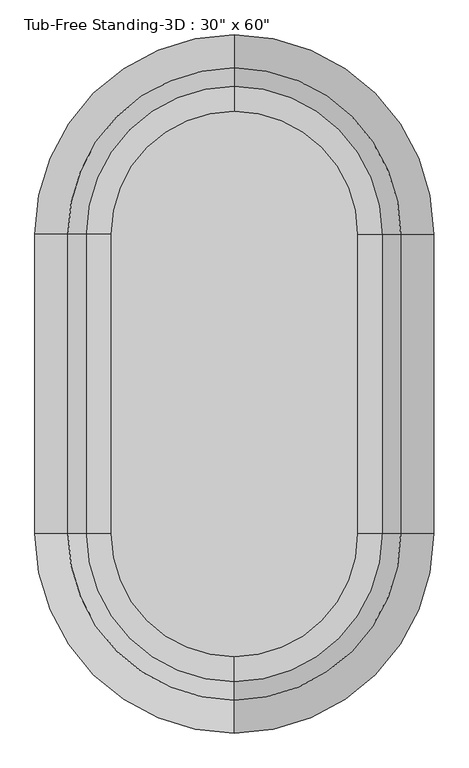
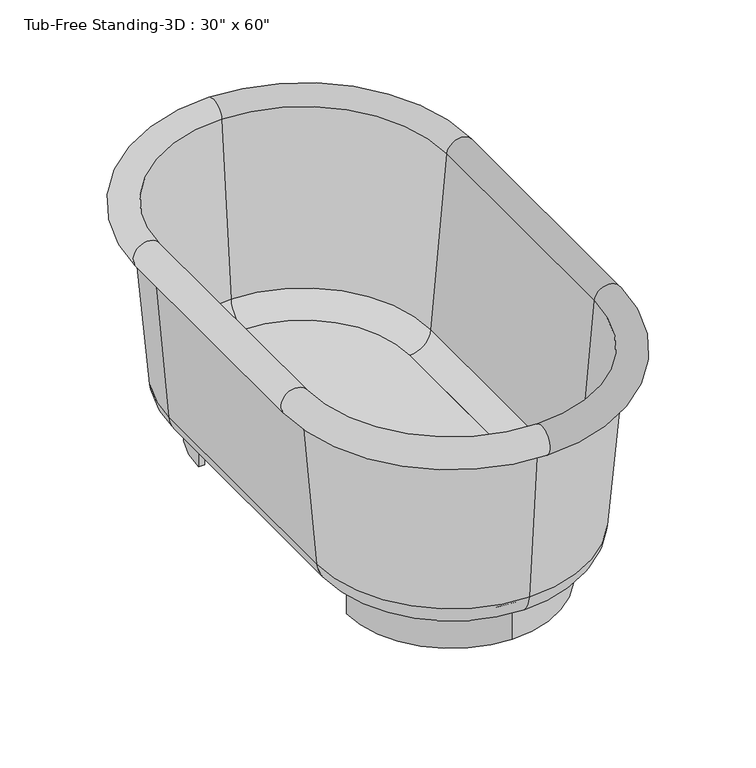
"""IFC4 building model written with IfcOpenShell, lengths in millimetres: flow terminal geometry."""

from ifc_helpers import new_model, si_unit, point, frame, frame_2d, origin, origin_with_axes, place, context, project, spatial, polyline, circle_curve, ellipse_curve, trimmed, segment, composite_curve, outline, extrude, source, transform, mapped, element, save
from ifc_brep_helpers import plane_surface, cylinder_surface, revolved_surface, advanced_brep


def flow_terminal_f143e1fa(model_context):
    return source(origin(), model_context, "Body", "SolidModel", [
        extrude(outline(composite_curve([segment(trimmed(circle_curve(frame_2d((0.0, 228.6)), 177.8), [point((0.0, 406.4))], [point((-177.8, 228.6))], True, "CARTESIAN"), True, "CONTINUOUS"), segment(polyline([(-177.8, 228.6), (-188.0824236, 228.6)]), True, "CONTINUOUS"), segment(trimmed(circle_curve(frame_2d((0.0, 228.6)), 188.0824236), [point((-188.0824236, 228.6))], [point((0.0, 416.6824236))], False, "CARTESIAN"), True, "CONTINUOUS"), segment(trimmed(circle_curve(frame_2d((0.0, 228.6)), 188.0824236), [point((0.0, 416.6824236))], [point((188.0824236, 228.6))], False, "CARTESIAN"), True, "CONTINUOUS"), segment(polyline([(188.0824236, 228.6), (177.8, 228.6)]), True, "CONTINUOUS"), segment(trimmed(circle_curve(frame_2d((0.0, 228.6)), 177.8), [point((177.8, 228.6))], [point((0.0, 406.4))], True, "CARTESIAN"), True, "CONTINUOUS")], self_intersect=False)), origin_with_axes(), (0.0, 0.0, 1.0), 63.5),
        extrude(outline(composite_curve([segment(trimmed(circle_curve(frame_2d((0.0, -228.6)), 188.0824236), [point((0.0, -416.6824236))], [point((-188.0824236, -228.6))], False, "CARTESIAN"), True, "CONTINUOUS"), segment(polyline([(-188.0824236, -228.6), (-177.8, -228.6)]), True, "CONTINUOUS"), segment(trimmed(circle_curve(frame_2d((0.0, -228.6)), 177.8), [point((-177.8, -228.6))], [point((0.0, -406.4))], True, "CARTESIAN"), True, "CONTINUOUS"), segment(trimmed(circle_curve(frame_2d((0.0, -228.6)), 177.8), [point((0.0, -406.4))], [point((177.8, -228.6))], True, "CARTESIAN"), True, "CONTINUOUS"), segment(polyline([(177.8, -228.6), (188.0824236, -228.6)]), True, "CONTINUOUS"), segment(trimmed(circle_curve(frame_2d((0.0, -228.6)), 188.0824236), [point((188.0824236, -228.6))], [point((0.0, -416.6824236))], False, "CARTESIAN"), True, "CONTINUOUS")], self_intersect=False)), origin_with_axes(), (0.0, 0.0, 1.0), 63.5),
        extrude(outline(composite_curve([segment(polyline([(-188.0824236, -228.6), (-188.0824236, 228.6)]), True, "CONTINUOUS"), segment(trimmed(circle_curve(frame_2d((0.0, 228.6)), 188.0824236), [point((-188.0824236, 228.6))], [point((0.0, 416.6824236))], False, "CARTESIAN"), True, "CONTINUOUS"), segment(trimmed(circle_curve(frame_2d((0.0, 228.6)), 188.0824236), [point((0.0, 416.6824236))], [point((188.0824236, 228.6))], False, "CARTESIAN"), True, "CONTINUOUS"), segment(polyline([(188.0824236, 228.6), (188.0824236, -228.6)]), True, "CONTINUOUS"), segment(trimmed(circle_curve(frame_2d((0.0, -228.6)), 188.0824236), [point((188.0824236, -228.6))], [point((0.0, -416.6824236))], False, "CARTESIAN"), True, "CONTINUOUS"), segment(trimmed(circle_curve(frame_2d((0.0, -228.6)), 188.0824236), [point((0.0, -416.6824236))], [point((-188.0824236, -228.6))], False, "CARTESIAN"), True, "CONTINUOUS")], self_intersect=False)), frame((0.0, 0.0, 63.5), z_axis=(0.0, 0.0, 1.0), x_axis=(1.0, 0.0, 0.0)), (0.0, 0.0, 1.0), 15.08125),
        advanced_brep(
        [(0.0, -495.3, 406.4), (266.7, -228.6, 406.4), (279.4, -228.6, 406.4), (0.0, -508.0, 406.4), (0.0, -469.5045038, 111.5561295), (240.9045038, -228.6, 111.5561295), (0.0, -416.6824236, 63.1536107), (188.0824236, -228.6, 63.1536107), (0.0, -416.6824236, 78.0774627), (188.0824236, -228.6, 78.0774627), (0.0, -454.6374416, 112.8568289), (226.0374416, -228.6, 112.8568289), (0.0, -482.8561556, 435.3982063), (254.2561556, -228.6, 435.3982063), (-266.7, -228.6, 406.4), (-279.4, -228.6, 406.4), (-240.9045038, -228.6, 111.5561295), (-188.0824236, -228.6, 63.1536107), (-188.0824236, -228.6, 78.0774627), (-226.0374416, -228.6, 112.8568289), (-254.2561556, -228.6, 435.3982063), (-279.4, 228.6, 406.4), (-266.7, 228.6, 406.4), (-240.9045038, 228.6, 111.5561295), (-188.0824236, 228.6, 63.1536107), (-188.0824236, 228.6, 78.0774627), (-226.0374416, 228.6, 112.8568289), (-254.2561556, 228.6, 435.3982063), (0.0, 495.3, 406.4), (0.0, 508.0, 406.4), (0.0, 469.5045038, 111.5561295), (0.0, 416.6824236, 63.1536107), (0.0, 416.6824236, 78.0774627), (0.0, 454.6374416, 112.8568289), (0.0, 482.8561556, 435.3982063), (266.7, 228.6, 406.4), (279.4, 228.6, 406.4), (240.9045038, 228.6, 111.5561295), (188.0824236, 228.6, 63.1536107), (188.0824236, 228.6, 78.0774627), (226.0374416, 228.6, 112.8568289), (254.2561556, 228.6, 435.3982063)],
        [
            (0, 1, circle_curve(frame((0.0, -228.6, 406.4), z_axis=(0.0, 0.0, 1.0), x_axis=(1.0, 0.0, 0.0)), 266.7)),
            (1, 2),
            (2, 3, circle_curve(frame((0.0, -228.6, 406.4), z_axis=(0.0, 0.0, -1.0), x_axis=(1.0, 0.0, 0.0)), 279.4)),
            (3, 0),
            (4, 5, circle_curve(frame((0.0, -228.6, 111.5561295), z_axis=(0.0, 0.0, 1.0), x_axis=(1.0, 0.0, 0.0)), 240.9045038)),
            (5, 1),
            (0, 4),
            (6, 7, circle_curve(frame((0.0, -228.6, 63.1536107), z_axis=(0.0, 0.0, 1.0), x_axis=(1.0, 0.0, 0.0)), 188.0824236)),
            (7, 5, circle_curve(frame((188.0824236, -228.6, 116.1774627), z_axis=(0.0, -1.0, 0.0), x_axis=(1.0, 0.0, 0.0)), 53.023852)),
            (4, 6, circle_curve(frame((0.0, -416.6824236, 116.1774627), z_axis=(1.0, 0.0, 0.0), x_axis=(0.0, -1.0, 0.0)), 53.023852)),
            (8, 9, circle_curve(frame((0.0, -228.6, 78.0774627), z_axis=(0.0, 0.0, 1.0), x_axis=(1.0, 0.0, 0.0)), 188.0824236)),
            (9, 7),
            (6, 8),
            (10, 11, circle_curve(frame((0.0, -228.6, 112.8568289), z_axis=(0.0, 0.0, 1.0), x_axis=(1.0, 0.0, 0.0)), 226.0374416)),
            (11, 9, circle_curve(frame((188.0824236, -228.6, 116.1774627), z_axis=(0.0, 1.0, 0.0), x_axis=(1.0, 0.0, 0.0)), 38.1)),
            (8, 10, circle_curve(frame((0.0, -416.6824236, 116.1774627), z_axis=(-1.0, 0.0, 0.0), x_axis=(0.0, -1.0, 0.0)), 38.1)),
            (12, 13, circle_curve(frame((0.0, -228.6, 435.3982063), z_axis=(0.0, 0.0, 1.0), x_axis=(1.0, 0.0, 0.0)), 254.2561556)),
            (13, 11),
            (10, 12),
            (2, 13, circle_curve(frame((279.4, -228.6, 431.8), z_axis=(0.0, -1.0, 0.0), x_axis=(1.0, 0.0, 0.0)), 25.4)),
            (12, 3, circle_curve(frame((0.0, -508.0, 431.8), z_axis=(1.0, 0.0, 0.0), x_axis=(0.0, -1.0, 0.0)), 25.4)),
            (14, 0, circle_curve(frame((0.0, -228.6, 406.4), z_axis=(0.0, 0.0, 1.0), x_axis=(0.0, -1.0, 0.0)), 266.7)),
            (3, 15, circle_curve(frame((0.0, -228.6, 406.4), z_axis=(0.0, 0.0, -1.0), x_axis=(0.0, -1.0, 0.0)), 279.4)),
            (15, 14),
            (16, 4, circle_curve(frame((0.0, -228.6, 111.5561295), z_axis=(0.0, 0.0, 1.0), x_axis=(0.0, -1.0, 0.0)), 240.9045038)),
            (14, 16),
            (17, 6, circle_curve(frame((0.0, -228.6, 63.1536107), z_axis=(0.0, 0.0, 1.0), x_axis=(0.0, -1.0, 0.0)), 188.0824236)),
            (16, 17, circle_curve(frame((-188.0824236, -228.6, 116.1774627), z_axis=(0.0, -1.0, 0.0), x_axis=(-1.0, 0.0, 0.0)), 53.023852)),
            (18, 8, circle_curve(frame((0.0, -228.6, 78.0774627), z_axis=(0.0, 0.0, 1.0), x_axis=(0.0, -1.0, 0.0)), 188.0824236)),
            (17, 18),
            (19, 10, circle_curve(frame((0.0, -228.6, 112.8568289), z_axis=(0.0, 0.0, 1.0), x_axis=(0.0, -1.0, 0.0)), 226.0374416)),
            (18, 19, circle_curve(frame((-188.0824236, -228.6, 116.1774627), z_axis=(0.0, 1.0, 0.0), x_axis=(-1.0, 0.0, 0.0)), 38.1)),
            (20, 12, circle_curve(frame((0.0, -228.6, 435.3982063), z_axis=(0.0, 0.0, 1.0), x_axis=(0.0, -1.0, 0.0)), 254.2561556)),
            (19, 20),
            (20, 15, circle_curve(frame((-279.4, -228.6, 431.8), z_axis=(0.0, -1.0, 0.0), x_axis=(-1.0, 0.0, 0.0)), 25.4)),
            (15, 21),
            (21, 22),
            (22, 14),
            (22, 23),
            (23, 16),
            (23, 24, circle_curve(frame((-188.0824236, 228.6, 116.1774627), z_axis=(0.0, -1.0, 0.0), x_axis=(-1.0, 0.0, 0.0)), 53.023852)),
            (24, 17),
            (24, 25),
            (25, 18),
            (25, 26, circle_curve(frame((-188.0824236, 228.6, 116.1774627), z_axis=(0.0, 1.0, 0.0), x_axis=(-1.0, 0.0, 0.0)), 38.1)),
            (26, 19),
            (26, 27),
            (27, 20),
            (27, 21, circle_curve(frame((-279.4, 228.6, 431.8), z_axis=(0.0, -1.0, 0.0), x_axis=(-1.0, 0.0, 0.0)), 25.4)),
            (28, 22, circle_curve(frame((0.0, 228.6, 406.4), z_axis=(0.0, 0.0, 1.0), x_axis=(-1.0, 0.0, 0.0)), 266.7)),
            (21, 29, circle_curve(frame((0.0, 228.6, 406.4), z_axis=(0.0, 0.0, -1.0), x_axis=(-1.0, 0.0, 0.0)), 279.4)),
            (29, 28),
            (30, 23, circle_curve(frame((0.0, 228.6, 111.5561295), z_axis=(0.0, 0.0, 1.0), x_axis=(-1.0, 0.0, 0.0)), 240.9045038)),
            (28, 30),
            (31, 24, circle_curve(frame((0.0, 228.6, 63.1536107), z_axis=(0.0, 0.0, 1.0), x_axis=(-1.0, 0.0, 0.0)), 188.0824236)),
            (30, 31, circle_curve(frame((0.0, 416.6824236, 116.1774627), z_axis=(-1.0, 0.0, 0.0), x_axis=(0.0, 1.0, 0.0)), 53.023852)),
            (32, 25, circle_curve(frame((0.0, 228.6, 78.0774627), z_axis=(0.0, 0.0, 1.0), x_axis=(-1.0, 0.0, 0.0)), 188.0824236)),
            (31, 32),
            (33, 26, circle_curve(frame((0.0, 228.6, 112.8568289), z_axis=(0.0, 0.0, 1.0), x_axis=(-1.0, 0.0, 0.0)), 226.0374416)),
            (32, 33, circle_curve(frame((0.0, 416.6824236, 116.1774627), z_axis=(1.0, 0.0, 0.0), x_axis=(0.0, 1.0, 0.0)), 38.1)),
            (34, 27, circle_curve(frame((0.0, 228.6, 435.3982063), z_axis=(0.0, 0.0, 1.0), x_axis=(-1.0, 0.0, 0.0)), 254.2561556)),
            (33, 34),
            (34, 29, circle_curve(frame((0.0, 508.0, 431.8), z_axis=(-1.0, 0.0, 0.0), x_axis=(0.0, 1.0, 0.0)), 25.4)),
            (35, 28, circle_curve(frame((0.0, 228.6, 406.4), z_axis=(0.0, 0.0, 1.0), x_axis=(0.0, 1.0, 0.0)), 266.7)),
            (29, 36, circle_curve(frame((0.0, 228.6, 406.4), z_axis=(0.0, 0.0, -1.0), x_axis=(0.0, 1.0, 0.0)), 279.4)),
            (36, 35),
            (37, 30, circle_curve(frame((0.0, 228.6, 111.5561295), z_axis=(0.0, 0.0, 1.0), x_axis=(0.0, 1.0, 0.0)), 240.9045038)),
            (35, 37),
            (38, 31, circle_curve(frame((0.0, 228.6, 63.1536107), z_axis=(0.0, 0.0, 1.0), x_axis=(0.0, 1.0, 0.0)), 188.0824236)),
            (37, 38, circle_curve(frame((188.0824236, 228.6, 116.1774627), z_axis=(0.0, 1.0, 0.0), x_axis=(1.0, 0.0, 0.0)), 53.023852)),
            (39, 32, circle_curve(frame((0.0, 228.6, 78.0774627), z_axis=(0.0, 0.0, 1.0), x_axis=(0.0, 1.0, 0.0)), 188.0824236)),
            (38, 39),
            (40, 33, circle_curve(frame((0.0, 228.6, 112.8568289), z_axis=(0.0, 0.0, 1.0), x_axis=(0.0, 1.0, 0.0)), 226.0374416)),
            (39, 40, circle_curve(frame((188.0824236, 228.6, 116.1774627), z_axis=(0.0, -1.0, 0.0), x_axis=(1.0, 0.0, 0.0)), 38.1)),
            (41, 34, circle_curve(frame((0.0, 228.6, 435.3982063), z_axis=(0.0, 0.0, 1.0), x_axis=(0.0, 1.0, 0.0)), 254.2561556)),
            (40, 41),
            (41, 36, circle_curve(frame((279.4, 228.6, 431.8), z_axis=(0.0, 1.0, 0.0), x_axis=(1.0, 0.0, 0.0)), 25.4)),
            (36, 2),
            (1, 35),
            (5, 37),
            (7, 38),
            (9, 39),
            (11, 40),
            (13, 41),
        ],
        [
            plane_surface(frame((0.0, -228.6, 406.4), z_axis=(0.0, 0.0, -1.0), x_axis=(1.0, 0.0, 0.0))),
            revolved_surface(polyline([(266.7, -228.6, 406.4), (240.9045038, -228.6, 111.5561295)]), (0.0, -228.6, 431.8), (0.0, 0.0, -1.0)),
            revolved_surface(trimmed(ellipse_curve(frame((188.0824236, -228.6, 116.1774627), z_axis=(0.0, 1.0, 0.0), x_axis=(1.0, 0.0, 0.0)), 53.023852, 53.023852), [point((240.9045038, -228.6, 111.5561295))], [point((188.0824236, -228.6, 63.1536107))], True, "CARTESIAN"), (0.0, -228.6, 431.8), (0.0, 0.0, -1.0)),
            revolved_surface(polyline([(188.0824236, -228.6, 63.1536107), (188.0824236, -228.6, 78.07746270000001)]), (0.0, -228.6, 431.8), (0.0, 0.0, -1.0)),
            revolved_surface(trimmed(ellipse_curve(frame((188.0824236, -228.6, 116.1774627), z_axis=(0.0, -1.0, 0.0), x_axis=(1.0, 0.0, 0.0)), 38.1, 38.1), [point((188.0824236, -228.6, 78.0774627))], [point((226.0374416, -228.6, 112.8568289))], True, "CARTESIAN"), (0.0, -228.6, 431.8), (0.0, 0.0, -1.0)),
            revolved_surface(polyline([(226.0374416, -228.6, 112.8568289), (254.2561556, -228.6, 435.3982063)]), (0.0, -228.6, 431.8), (0.0, 0.0, -1.0)),
            revolved_surface(trimmed(ellipse_curve(frame((279.4, -228.6, 431.8), z_axis=(0.0, 1.0, 0.0), x_axis=(1.0, 0.0, 0.0)), 25.4, 25.4), [point((254.2561556, -228.6, 435.3982063))], [point((279.4, -228.6, 406.4))], True, "CARTESIAN"), (0.0, -228.6, 431.8), (0.0, 0.0, -1.0)),
            plane_surface(frame((0.0, -228.6, 406.4), z_axis=(0.0, 0.0, -1.0), x_axis=(0.0, -1.0, 0.0))),
            revolved_surface(polyline([(0.0, -495.3, 406.4), (0.0, -469.5045038, 111.5561295)]), (0.0, -228.6, 431.8), (0.0, 0.0, -1.0)),
            revolved_surface(trimmed(ellipse_curve(frame((0.0, -416.6824236, 116.1774627), z_axis=(1.0, 0.0, 0.0), x_axis=(0.0, -1.0, 0.0)), 53.023852, 53.023852), [point((0.0, -469.5045038, 111.5561295))], [point((0.0, -416.6824236, 63.1536107))], True, "CARTESIAN"), (0.0, -228.6, 431.8), (0.0, 0.0, -1.0)),
            revolved_surface(polyline([(0.0, -416.6824236, 63.1536107), (0.0, -416.6824236, 78.07746270000001)]), (0.0, -228.6, 431.8), (0.0, 0.0, -1.0)),
            revolved_surface(trimmed(ellipse_curve(frame((0.0, -416.6824236, 116.1774627), z_axis=(-1.0, 0.0, 0.0), x_axis=(0.0, -1.0, 0.0)), 38.1, 38.1), [point((0.0, -416.6824236, 78.0774627))], [point((0.0, -454.6374416, 112.8568289))], True, "CARTESIAN"), (0.0, -228.6, 431.8), (0.0, 0.0, -1.0)),
            revolved_surface(polyline([(0.0, -454.6374416, 112.8568289), (0.0, -482.8561556, 435.3982063)]), (0.0, -228.6, 431.8), (0.0, 0.0, -1.0)),
            revolved_surface(trimmed(ellipse_curve(frame((0.0, -508.0, 431.8), z_axis=(1.0, 0.0, 0.0), x_axis=(0.0, -1.0, 0.0)), 25.4, 25.4), [point((0.0, -482.8561556, 435.3982063))], [point((0.0, -508.0, 406.4))], True, "CARTESIAN"), (0.0, -228.6, 431.8), (0.0, 0.0, -1.0)),
            plane_surface(frame((-279.4, -228.6, 406.4), z_axis=(0.0, 0.0, -1.0), x_axis=(0.0, 1.0, 0.0))),
            plane_surface(frame((-266.7, -228.6, 406.4), z_axis=(-0.9961946980917455, 0.0, -0.08715574274765882), x_axis=(0.0, 1.0, 0.0))),
            cylinder_surface(frame((-188.0824236, -228.6, 116.1774627), z_axis=(0.0, -1.0, 0.0), x_axis=(-1.0, 0.0, 0.0)), 53.023852),
            plane_surface(frame((-188.0824236, -228.6, 63.1536107), z_axis=(1.0, 0.0, 0.0), x_axis=(0.0, 1.0, 0.0))),
            revolved_surface(polyline([(-226.1824236, 228.6, 116.1774627), (-226.1824236, -228.6, 116.1774627)]), (-188.0824236, -228.6, 116.1774627), (0.0, 1.0, 0.0)),
            plane_surface(frame((-226.0374416, -228.6, 112.8568289), z_axis=(0.9961946980917457, 0.0, 0.08715574274765679), x_axis=(0.0, 1.0, 0.0))),
            cylinder_surface(frame((-279.4, -228.6, 431.8), z_axis=(0.0, -1.0, 0.0), x_axis=(-1.0, 0.0, 0.0)), 25.4),
            plane_surface(frame((0.0, 228.6, 406.4), z_axis=(0.0, 0.0, -1.0), x_axis=(-1.0, 0.0, 0.0))),
            revolved_surface(polyline([(-266.7, 228.6, 406.4), (-240.9045038, 228.6, 111.5561295)]), (0.0, 228.6, 431.8), (0.0, 0.0, -1.0)),
            revolved_surface(trimmed(ellipse_curve(frame((-188.0824236, 228.6, 116.1774627), z_axis=(0.0, -1.0, 0.0), x_axis=(-1.0, 0.0, 0.0)), 53.023852, 53.023852), [point((-240.9045038, 228.6, 111.5561295))], [point((-188.0824236, 228.6, 63.1536107))], True, "CARTESIAN"), (0.0, 228.6, 431.8), (0.0, 0.0, -1.0)),
            revolved_surface(polyline([(-188.0824236, 228.6, 63.1536107), (-188.0824236, 228.6, 78.07746270000001)]), (0.0, 228.6, 431.8), (0.0, 0.0, -1.0)),
            revolved_surface(trimmed(ellipse_curve(frame((-188.0824236, 228.6, 116.1774627), z_axis=(0.0, 1.0, 0.0), x_axis=(-1.0, 0.0, 0.0)), 38.1, 38.1), [point((-188.0824236, 228.6, 78.0774627))], [point((-226.0374416, 228.6, 112.8568289))], True, "CARTESIAN"), (0.0, 228.6, 431.8), (0.0, 0.0, -1.0)),
            revolved_surface(polyline([(-226.0374416, 228.6, 112.8568289), (-254.2561556, 228.6, 435.3982063)]), (0.0, 228.6, 431.8), (0.0, 0.0, -1.0)),
            revolved_surface(trimmed(ellipse_curve(frame((-279.4, 228.6, 431.8), z_axis=(0.0, -1.0, 0.0), x_axis=(-1.0, 0.0, 0.0)), 25.4, 25.4), [point((-254.2561556, 228.6, 435.3982063))], [point((-279.4, 228.6, 406.4))], True, "CARTESIAN"), (0.0, 228.6, 431.8), (0.0, 0.0, -1.0)),
            plane_surface(frame((0.0, 228.6, 406.4), z_axis=(0.0, 0.0, -1.0), x_axis=(0.0, 1.0, 0.0))),
            revolved_surface(polyline([(0.0, 495.3, 406.4), (0.0, 469.5045038, 111.5561295)]), (0.0, 228.6, 431.8), (0.0, 0.0, -1.0)),
            revolved_surface(trimmed(ellipse_curve(frame((0.0, 416.6824236, 116.1774627), z_axis=(-1.0, 0.0, 0.0), x_axis=(0.0, 1.0, 0.0)), 53.023852, 53.023852), [point((0.0, 469.5045038, 111.5561295))], [point((0.0, 416.6824236, 63.1536107))], True, "CARTESIAN"), (0.0, 228.6, 431.8), (0.0, 0.0, -1.0)),
            revolved_surface(polyline([(0.0, 416.6824236, 63.1536107), (0.0, 416.6824236, 78.07746270000001)]), (0.0, 228.6, 431.8), (0.0, 0.0, -1.0)),
            revolved_surface(trimmed(ellipse_curve(frame((0.0, 416.6824236, 116.1774627), z_axis=(1.0, 0.0, 0.0), x_axis=(0.0, 1.0, 0.0)), 38.1, 38.1), [point((0.0, 416.6824236, 78.0774627))], [point((0.0, 454.6374416, 112.8568289))], True, "CARTESIAN"), (0.0, 228.6, 431.8), (0.0, 0.0, -1.0)),
            revolved_surface(polyline([(0.0, 454.6374416, 112.8568289), (0.0, 482.8561556, 435.3982063)]), (0.0, 228.6, 431.8), (0.0, 0.0, -1.0)),
            revolved_surface(trimmed(ellipse_curve(frame((0.0, 508.0, 431.8), z_axis=(-1.0, 0.0, 0.0), x_axis=(0.0, 1.0, 0.0)), 25.4, 25.4), [point((0.0, 482.8561556, 435.3982063))], [point((0.0, 508.0, 406.4))], True, "CARTESIAN"), (0.0, 228.6, 431.8), (0.0, 0.0, -1.0)),
            plane_surface(frame((279.4, 228.6, 406.4), z_axis=(0.0, 0.0, -1.0), x_axis=(0.0, -1.0, 0.0))),
            plane_surface(frame((266.7, 228.6, 406.4), z_axis=(0.9961946980917455, 0.0, -0.08715574274765882), x_axis=(0.0, -1.0, 0.0))),
            cylinder_surface(frame((188.0824236, 228.6, 116.1774627), z_axis=(0.0, 1.0, 0.0), x_axis=(1.0, 0.0, 0.0)), 53.023852),
            plane_surface(frame((188.0824236, 228.6, 63.1536107), z_axis=(-1.0, 0.0, 0.0), x_axis=(0.0, -1.0, 0.0))),
            revolved_surface(polyline([(226.1824236, -228.6, 116.1774627), (226.1824236, 228.6, 116.1774627)]), (188.0824236, 228.6, 116.1774627), (0.0, -1.0, 0.0)),
            plane_surface(frame((226.0374416, 228.6, 112.8568289), z_axis=(-0.9961946980917458, 0.0, 0.0871557427476568), x_axis=(0.0, -1.0, 0.0))),
            cylinder_surface(frame((279.4, 228.6, 431.8), z_axis=(0.0, 1.0, 0.0), x_axis=(1.0, 0.0, 0.0)), 25.4),
        ],
        [
            (0, [[1, 2, 3, 4]]),
            (1, [[5, 6, -1, 7]]),
            (2, [[8, 9, -5, 10]]),
            (3, [[11, 12, -8, 13]]),
            (4, [[14, 15, -11, 16]]),
            (5, [[17, 18, -14, 19]]),
            (6, [[-3, 20, -17, 21]]),
            (7, [[22, -4, 23, 24]]),
            (8, [[25, -7, -22, 26]]),
            (9, [[27, -10, -25, 28]]),
            (10, [[29, -13, -27, 30]]),
            (11, [[31, -16, -29, 32]]),
            (12, [[33, -19, -31, 34]]),
            (13, [[-23, -21, -33, 35]]),
            (14, [[-24, 36, 37, 38]]),
            (15, [[-26, -38, 39, 40]]),
            (16, [[-28, -40, 41, 42]]),
            (17, [[-30, -42, 43, 44]]),
            (18, [[-32, -44, 45, 46]]),
            (19, [[-34, -46, 47, 48]]),
            (20, [[-35, -48, 49, -36]]),
            (21, [[50, -37, 51, 52]]),
            (22, [[53, -39, -50, 54]]),
            (23, [[55, -41, -53, 56]]),
            (24, [[57, -43, -55, 58]]),
            (25, [[59, -45, -57, 60]]),
            (26, [[61, -47, -59, 62]]),
            (27, [[-51, -49, -61, 63]]),
            (28, [[64, -52, 65, 66]]),
            (29, [[67, -54, -64, 68]]),
            (30, [[69, -56, -67, 70]]),
            (31, [[71, -58, -69, 72]]),
            (32, [[73, -60, -71, 74]]),
            (33, [[75, -62, -73, 76]]),
            (34, [[-65, -63, -75, 77]]),
            (35, [[-66, 78, -2, 79]]),
            (36, [[-68, -79, -6, 80]]),
            (37, [[-70, -80, -9, 81]]),
            (38, [[-72, -81, -12, 82]]),
            (39, [[-74, -82, -15, 83]]),
            (40, [[-76, -83, -18, 84]]),
            (41, [[-77, -84, -20, -78]]),
        ],
    ),
    ])


if __name__ == "__main__":
    model = new_model("IFC4")
    model_context = context("Model", 3, world=origin())
    ifc_project = project(units=[si_unit("LENGTHUNIT", "METRE", prefix="MILLI")], contexts=[model_context])
    site = spatial("IfcSite", under=ifc_project)
    building = spatial("IfcBuilding", under=site)
    placement = place(None, origin())
    flow_terminal_shape = flow_terminal_f143e1fa(model_context)
    element("IfcFlowTerminal", 1, ObjectType="Tub-Free Standing-3D : 30\" x 60\"", at=placement, inside=building, context=model_context, shape_type="MappedRepresentation", body=[
        mapped(flow_terminal_shape, transform((0.0, 0.0, 0.0), x_axis=(1.0, 0.0, 0.0), y_axis=(0.0, 1.0, 0.0), z_axis=(0.0, 0.0, 1.0))),
    ])
    save(model, "model.ifc")

# Revit data of these elements
# Type "Tub-Free Standing-3D : 30\" x 60\""
#   Assembly Code = "D2010110"
#   Height = 1' - 6"
#   Length = 3' - 6"
#   Width = 2' - 0"
#   Tub Material = Porcelain, Ivory
#   Default Elevation = 0
# Element 1 (IfcFlowTerminal, "Tub-Free Standing-3D : 30\" x 60\"")
#   Materials on its faces: "Porcelain, Ivory"
# Materials
#   "Porcelain, Ivory": class "Ceramic", colour RGB 247 247 239, transparency 0, Description = "Porcelain, ivory", Cost = 0
